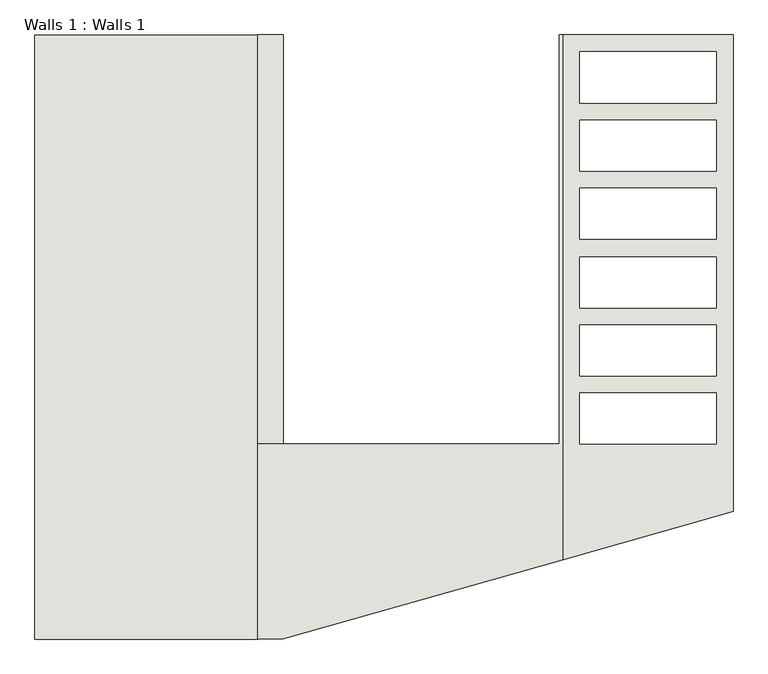
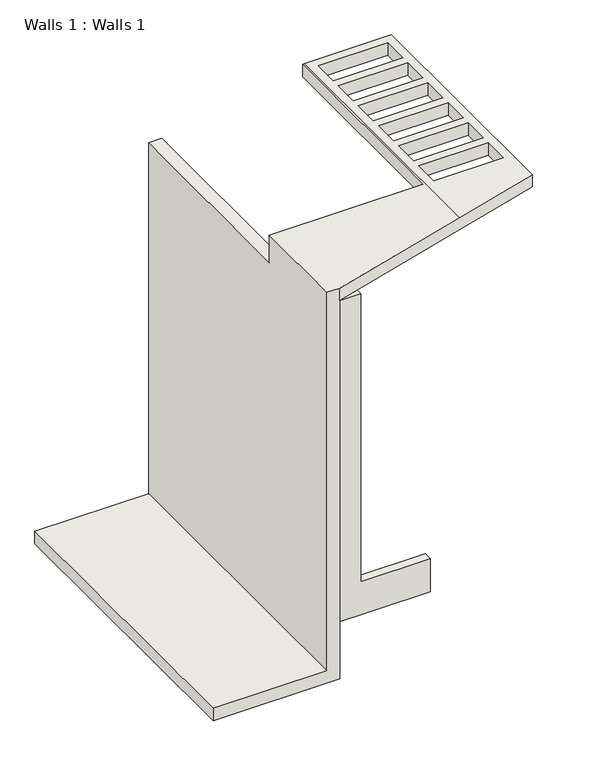
"""IFC4 building model written with IfcOpenShell, lengths in millimetres: wall geometry, Walls 1 : Walls 1."""

from ifc_helpers import new_model, si_unit, frame, origin, place, context, project, spatial, polyline, outline, extrude, faceted_brep, source, transform, mapped, element, save


def walls_1_walls_1_280b9ad2(model_context):
    return source(origin(), model_context, "Body", "SolidModel", [
        extrude(outline(polyline([(600.0, -9917.6792561), (600.0, -11117.6792561), (5850.0, -11117.6792561), (5850.0, -11717.6792561), (0.0, -11717.6792561), (0.0, -9917.6792561), (600.0, -9917.6792561)])), frame((0.0, -6226.7197682, 0.0), z_axis=(0.0, 1.0, 0.0), x_axis=(0.0, 0.0, 1.0)), (0.0, 0.0, 1.0), 150.0),
        faceted_brep([(-12605.1792561, -7794.2197682, 7350.0), (-12605.1792561, -7794.2197682, 450.0), (-14567.6792561, -7794.2197682, 450.0), (-14567.6792561, -7794.2197682, 225.0), (-12380.1792561, -7794.2197682, 225.0), (-12380.1792561, -7794.2197682, 6850.0), (-12380.1792561, -7794.2197682, 7125.0), (-12380.1792561, -7794.2197682, 7350.0), (-9917.6792561, -2469.2197682, 7350.0), (-8417.6792561, -2469.2197682, 7350.0), (-8417.6792561, -2469.2197682, 7125.0), (-9917.6792561, -2469.2197682, 7125.0), (-9950.1792561, -2469.2197682, 7125.0), (-9950.1792561, -2469.2197682, 7350.0), (-12380.1792561, -2469.2197682, 225.0), (-14567.6792561, -2469.2197682, 225.0), (-14567.6792561, -2469.2197682, 450.0), (-12605.1792561, -2469.2197682, 450.0), (-12605.1792561, -2469.2197682, 6850.0), (-12380.1792561, -2469.2197682, 6850.0), (-9917.6792561, -7095.0872761, 7350.0), (-9950.1792561, -6076.7197682, 7350.0), (-12605.1792561, -6076.7197682, 7350.0), (-12605.1792561, -6076.7197682, 6850.0), (-12380.1792561, -6076.7197682, 6850.0), (-12380.1792561, -6076.7197682, 7125.0), (-9917.6792561, -7095.0872761, 7125.0), (-9950.1792561, -6076.7197682, 7125.0), (-8417.6792561, -6669.2197682, 7125.0), (-9767.6792561, -2619.2197682, 7125.0), (-9767.6792561, -3069.2197682, 7125.0), (-8567.6792561, -3069.2197682, 7125.0), (-8567.6792561, -2619.2197682, 7125.0), (-9767.6792561, -3219.2197682, 7125.0), (-9767.6792561, -3669.2197682, 7125.0), (-8567.6792561, -3669.2197682, 7125.0), (-8567.6792561, -3219.2197682, 7125.0), (-9767.6792561, -3819.2197682, 7125.0), (-9767.6792561, -4269.2197682, 7125.0), (-8567.6792561, -4269.2197682, 7125.0), (-8567.6792561, -3819.2197682, 7125.0), (-9767.6792561, -4426.7197682, 7125.0), (-9767.6792561, -4876.7197682, 7125.0), (-8567.6792561, -4876.7197682, 7125.0), (-8567.6792561, -4426.7197682, 7125.0), (-9767.6792561, -5026.7197682, 7125.0), (-9767.6792561, -5476.7197682, 7125.0), (-8567.6792561, -5476.7197682, 7125.0), (-8567.6792561, -5026.7197682, 7125.0), (-9767.6792561, -5626.7197682, 7125.0), (-9767.6792561, -6076.7197682, 7125.0), (-8567.6792561, -6076.7197682, 7125.0), (-8567.6792561, -5626.7197682, 7125.0), (-8417.6792561, -6669.2197682, 7350.0), (-9767.6792561, -3069.2197682, 7350.0), (-9767.6792561, -2619.2197682, 7350.0), (-8567.6792561, -2619.2197682, 7350.0), (-8567.6792561, -3069.2197682, 7350.0), (-9767.6792561, -3669.2197682, 7350.0), (-9767.6792561, -3219.2197682, 7350.0), (-8567.6792561, -3219.2197682, 7350.0), (-8567.6792561, -3669.2197682, 7350.0), (-9767.6792561, -4269.2197682, 7350.0), (-9767.6792561, -3819.2197682, 7350.0), (-8567.6792561, -3819.2197682, 7350.0), (-8567.6792561, -4269.2197682, 7350.0), (-9767.6792561, -4876.7197682, 7350.0), (-9767.6792561, -4426.7197682, 7350.0), (-8567.6792561, -4426.7197682, 7350.0), (-8567.6792561, -4876.7197682, 7350.0), (-9767.6792561, -5476.7197682, 7350.0), (-9767.6792561, -5026.7197682, 7350.0), (-8567.6792561, -5026.7197682, 7350.0), (-8567.6792561, -5476.7197682, 7350.0), (-9767.6792561, -6076.7197682, 7350.0), (-9767.6792561, -5626.7197682, 7350.0), (-8567.6792561, -5626.7197682, 7350.0), (-8567.6792561, -6076.7197682, 7350.0)], [[[0, 1, 2, 3, 4, 5, 6, 7]], [[8, 9, 10, 11, 12, 13]], [[14, 15, 16, 17, 18, 19]], [[0, 7, 20, 8, 13, 21, 22]], [[1, 0, 22, 23, 18, 17]], [[2, 1, 17, 16]], [[3, 2, 16, 15]], [[4, 3, 15, 14]], [[4, 14, 19, 24, 25, 6, 5]], [[12, 11, 26, 6, 25, 27]], [[11, 10, 28, 26], [29, 30, 31, 32], [33, 34, 35, 36], [37, 38, 39, 40], [41, 42, 43, 44], [45, 46, 47, 48], [49, 50, 51, 52]], [[10, 9, 53, 28]], [[9, 8, 20, 53], [54, 55, 56, 57], [58, 59, 60, 61], [62, 63, 64, 65], [66, 67, 68, 69], [70, 71, 72, 73], [74, 75, 76, 77]], [[23, 24, 19, 18]], [[27, 21, 13, 12]], [[24, 23, 22, 21, 27, 25]], [[54, 30, 29, 55]], [[55, 29, 32, 56]], [[56, 32, 31, 57]], [[30, 54, 57, 31]], [[58, 34, 33, 59]], [[59, 33, 36, 60]], [[60, 36, 35, 61]], [[34, 58, 61, 35]], [[62, 38, 37, 63]], [[63, 37, 40, 64]], [[64, 40, 39, 65]], [[38, 62, 65, 39]], [[66, 42, 41, 67]], [[67, 41, 44, 68]], [[68, 44, 43, 69]], [[42, 66, 69, 43]], [[70, 46, 45, 71]], [[71, 45, 48, 72]], [[72, 48, 47, 73]], [[46, 70, 73, 47]], [[74, 50, 49, 75]], [[75, 49, 52, 76]], [[76, 52, 51, 77]], [[50, 74, 77, 51]], [[7, 6, 26, 28, 53, 20]]]),
    ])


if __name__ == "__main__":
    model = new_model("IFC4")
    model_context = context("Model", 3, world=origin())
    ifc_project = project(units=[si_unit("LENGTHUNIT", "METRE", prefix="MILLI")], contexts=[model_context])
    site = spatial("IfcSite", under=ifc_project)
    building = spatial("IfcBuilding", under=site)
    placement = place(None, origin())
    walls_1_walls_1_shape = walls_1_walls_1_280b9ad2(model_context)
    element("IfcWall", 1, ObjectType="Walls 1 : Walls 1", at=placement, inside=building, context=model_context, shape_type="MappedRepresentation", body=[
        mapped(walls_1_walls_1_shape, transform((0.0, 0.0, 0.0), x_axis=(1.0, 0.0, 0.0), y_axis=(0.0, 1.0, 0.0), z_axis=(0.0, 0.0, 1.0))),
    ])
    save(model, "model.ifc")

# Revit data of these elements
# Element 1 (IfcWall, "Walls 1 : Walls 1")
#   Materials on its faces: "00-white plaster", "00-white plaster(2)"
# Materials
#   "00-white plaster": class "Masonry", colour RGB 244 244 244, transparency 0, Description = "Common brick", Cost = 0
#   "00-white plaster(2)": class "Masonry", colour RGB 20 28 51, transparency 0, Description = "Common brick", Cost = 0
